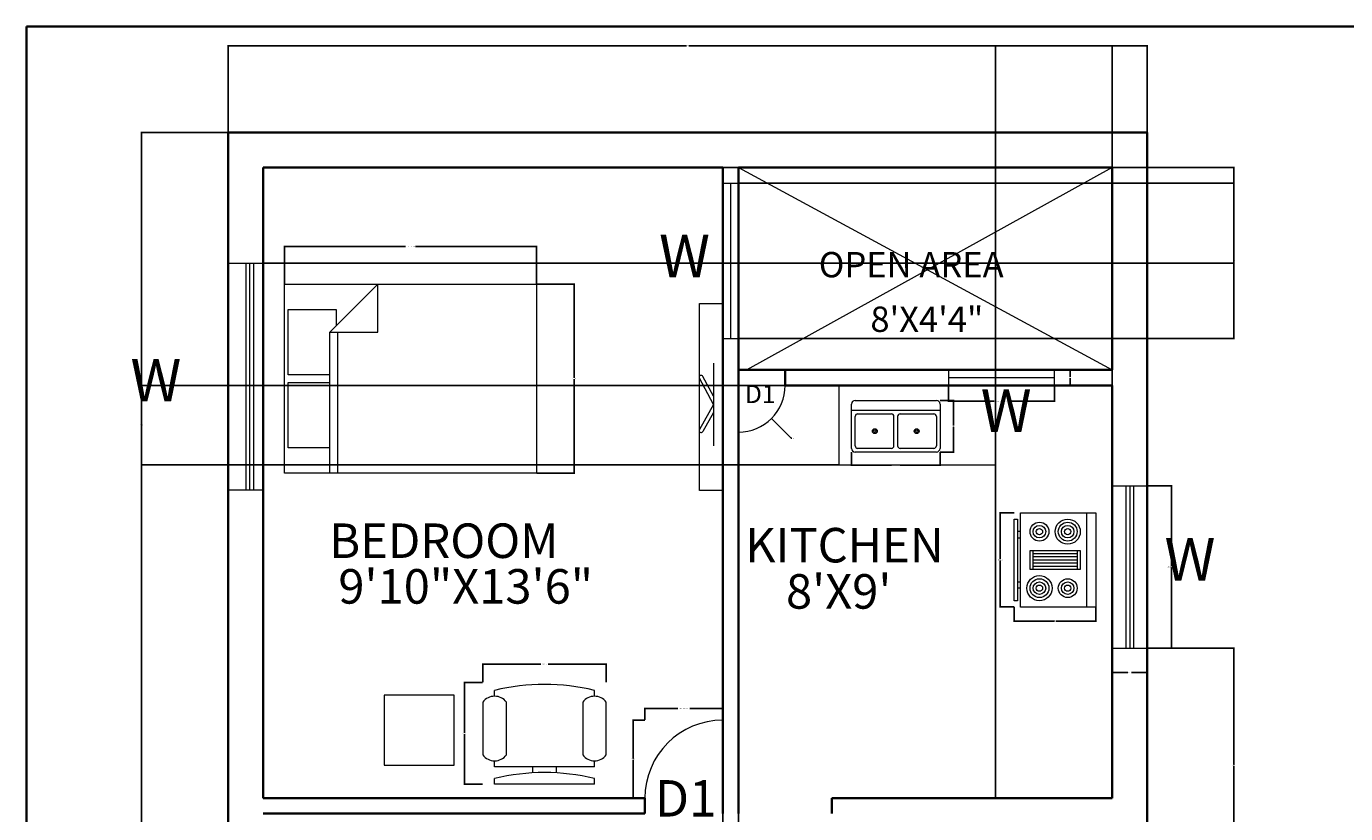
# Model space of a CAD drawing. Units: feet. Extents: x 38163 to 38841, y 65807 to 66292.
# Tile 2 of 3: x 38163 to 38502, y 66090 to 66292. Entities that reach past the tile are written whole.
import ezdxf

# ---------------------------------------------------------------- set-up
doc = ezdxf.new("R2010")
doc.units = ezdxf.units.FT
for name, color, linetype, lineweight in [('A-ANNO-DIMS', 2, 'Continuous', 18), ('A-ANNO-TEXT', 7, 'Continuous', 18), ('A-ANNO-TTLB', 7, 'Continuous', 35), ('A-AREA-IDEN', 7, 'Continuous', 18), ('A-DOOR', 4, 'Continuous', 18), ('A-EQPM', 8, 'Continuous', 18), ('A-FLOR-CASE', 9, 'Continuous', 18), ('A-FLOR-FIXT', 9, 'Continuous', 18), ('A-FLOR-OPEN', 8, 'Continuous', 13), ('A-FURN', 8, 'Continuous', 18), ('A-GLAZ', 4, 'Continuous', 13), ('A-WALL', 7, 'Continuous', 35)]:
    doc.layers.add(name, color=color, linetype=linetype, lineweight=lineweight)
doc.styles.get("Standard").update_dxf_attribs({"font": 'arial.ttf'})
doc.dimstyles.get("Standard").update_dxf_attribs({"dimtxt": 0.18, "dimasz": 0.18, "dimexe": 0.18, "dimexo": 0.0625, "dimgap": 0.09, "dimtad": 0, "dimtih": 1, "dimtoh": 1, "dimdec": 4, "dimzin": 0, "dimdsep": 46, "dimtxsty": 'Standard', "dimcen": 0.09, "dimadec": 0, "dimazin": 0, "dimtfac": 1, "dimtdec": 4, "dimtofl": 0, "dimtmove": 0, "dimatfit": 3, "dimfxl": 1, "dimtolj": 1, "dimtzin": 0, "dimarcsym": 0})

# ---------------------------------------------------------------- blocks, each defined once
blk = doc.blocks.new('Bed - Queen')
for p, q in [((0, -80.00003), (0, 0)), ((0, 0), (59.99999, 0)), ((59.99999, 0), (59.99999, -80.00003)), ((7.99999, -1.2), (28.79998, -1.2)), ((7.99999, -14.4), (7.99999, -1.2)), ((28.79998, -1.2), (28.79998, -14.4)), ((31.19999, -1.2), (51.99999, -1.2)), ((31.19999, -14.4), (31.19999, -1.2)), ((51.99999, -1.2), (51.99999, -16.4)), ((0, -14.4), (44.8, -14.4)), ((59.99999, -29.6), (44.8, -14.4)), ((44.8, -14.4), (44.8, -29.6)), ((51.99999, -16.4), (46.79936, -16.4)), ((44.8, -16.8), (0, -16.8)), ((44.8, -29.6), (59.99999, -29.6)), ((59.99999, -80.00003), (0, -80.00003))]:
    blk.add_line(p, q)
blk = doc.blocks.new('Chair - Desk')
for p, q in [((-8.5, 0), (-8.5, -1)), ((-8.5, 0), (8.5, 0)), ((8.5, 0), (8.5, -1)), ((-2, -3), (-2, -1.9355)), ((2, -1.9576), (2, -3)), ((-8.5, -3), (-8.5, -4)), ((-8.5, -3), (8.5, -3)), ((8.5, -3), (8.5, -4)), ((-10.5, -5), (-10.5, -14)), ((-6.5, -14), (-6.5, -5)), ((6.5, -5), (6.5, -14)), ((10.5, -14), (10.5, -5)), ((-8.5, -15), (-8.5, -16)), ((8.5, -15), (8.5, -16))]:
    blk.add_line(p, q)
for centre, radius, start, end in [((0, 34.625), 36.625, 256.5803, 283.4197), ((-8.5, -6.5), 2.5, 36.8699, 143.1301), ((8.5, -6.5), 2.5, 36.8699, 143.1301), ((-8.5, -12.5), 2.5, 216.8699, 323.1301), ((8.5, -12.5), 2.5, 216.8699, 323.1301), ((0, 19.625), 36.625, 256.5803, 283.4197)]:
    blk.add_arc(centre, radius, start, end)
blk = doc.blocks.new('Range-Oven - 30 in top')
for p, q in [((0, -3), (30, -3)), ((12, -6), (18, -6)), ((13, -20), (13, -6)), ((14, -6), (14, -20)), ((15, -20), (15, -6)), ((16, -6), (16, -20)), ((17, -20), (17, -6)), ((18, -20), (12, -20)), ((6, -24), (6, -25)), ((8, -25), (8, -24)), ((22, -25), (22, -24)), ((24, -24), (24, -25))]:
    blk.add_line(p, q)
for points in [[(0, -24), (0, 0), (30, 0), (30, -24)], [(12, -21), (12, -5), (18, -5), (18, -21)], [(2, -26), (2, -25), (28, -25), (28, -26)]]:
    blk.add_lwpolyline(points, close=True)
for centre, radius in [((6, -9), 4), ((6, -9), 3), ((6, -9), 2), ((6, -9), 1), ((24, -9), 3), ((24, -9), 2), ((24, -9), 1), ((6, -18), 3), ((6, -18), 2), ((24, -18), 4), ((24, -18), 3), ((24, -18), 2), ((6, -18), 1), ((24, -18), 1)]:
    blk.add_circle(centre, radius)
blk = doc.blocks.new('Sink-double - 36 in top')
for p, q in [((-18, -4), (18, -4)), ((-0.75, -18.5), (-0.75, -6.5)), ((0.75, -6.5), (0.75, -18.5))]:
    blk.add_line(p, q)
for points in [[(-16.5, 0), (16.5, 0)], [(-18, -19.5), (-18, -1.5)], [(18, -1.5), (18, -19.5)], [(-16.5, -18.5), (-16.5, -6.5)], [(-15.5, -5.5), (-1.75, -5.5)], [(1.75, -5.5), (15.5, -5.5)], [(16.5, -6.5), (16.5, -18.5)], [(16.5, -21), (-16.5, -21)], [(-1.75, -19.5), (-15.5, -19.5)], [(15.5, -19.5), (1.75, -19.5)]]:
    blk.add_lwpolyline(points)
for centre, radius in [((-8.5, -12.5), 1), ((-8.5, -12.5), 0.5), ((8.5, -12.5), 1), ((8.5, -12.5), 0.5)]:
    blk.add_circle(centre, radius)
for centre, radius, start, end in [((-16.5, -1.5), 1.5, 90, 180), ((16.5, -1.5), 1.5, 0, 90), ((-15.5, -6.5), 1, 90, 180), ((-1.75, -6.5), 1, 0, 90), ((1.75, -6.5), 1, 90, 180), ((15.5, -6.5), 1, 0, 90), ((-16.5, -19.5), 1.5, 180, 270), ((-15.5, -18.5), 1, 180, 270), ((-1.75, -18.5), 1, 270, 0), ((1.75, -18.5), 1, 180, 270), ((15.5, -18.5), 1, 270, 0), ((16.5, -19.5), 1.5, 270, 0)]:
    blk.add_arc(centre, radius, start, end)
blk = doc.blocks.new('DOOR-SWING-20')
blk.add_line((20, 0), (20, 20))
blk.add_arc((20, 0), 20, 90, 180)
blk = doc.blocks.new('TABLE-SQUARE')
for p, q in [((18, 18), (0, 18)), ((0, 18), (0, 0)), ((18, 0), (18, 18)), ((0, 0), (18, 0))]:
    blk.add_line(p, q)
blk = doc.blocks.new('TV-CONSOLE')
for p, q in [((0.06, 48), (6.06, 48)), ((0.06, 0), (0.06, 48)), ((6.06, 48), (6.06, 0)), ((3.68, 32.75), (3.68, 11.44)), ((3.68, 22.09), (0.06, 28.83)), ((3.68, 24.21), (0.94, 29.3)), ((3.68, 22.09), (0.06, 15.67)), ((3.68, 20.06), (0.93, 15.18)), ((6.06, 0), (0.06, 0))]:
    blk.add_line(p, q)
for centre, start, end in [((0.5, 29.07), 28.2522, 208.2522), ((0.5, 15.42), 150.6168, 330.6168)]:
    blk.add_arc(centre, 0.5, start, end)
blk = doc.blocks.new('WIN-SIDE-REAR')
for p, q in [((0, 41.67), (9, 41.67)), ((3.5, 41.67), (3.5, 0)), ((4.5, 41.67), (4.5, 0)), ((5.5, 41.67), (5.5, 0)), ((0, 0), (9, 0))]:
    blk.add_line(p, q)
blk = doc.blocks.new('WIN-LIGHTWELL')
for p, q in [((0, 0), (0, 4)), ((27.16, 0), (27.16, 4)), ((0, 2), (27.16, 2))]:
    blk.add_line(p, q)
blk = doc.blocks.new('LIGHTWELL-CROSS')
for p, q in [((0, 52), (96, 0)), ((96, 52), (2.18, 0))]:
    blk.add_line(p, q)
blk = doc.blocks.new('*D21')
at = {"layer": 'A-ANNO-DIMS', "color": 0, "lineweight": -2, "transparency": 16777216}
for p, q in [((38322.09, 66114.08), (38322.09, 66117.19)), ((38322.27, 66117.01), (38330.52, 66117.01)), ((38341.91, 66117.01), (38333.66, 66117.01)), ((38342.09, 66114.08), (38342.09, 66117.19))]:
    blk.add_line(p, q, dxfattribs=at)
at = {"layer": 'A-ANNO-DIMS', "color": 0, "transparency": 16777216}
for points in [[(38322.27, 66117.04), (38322.27, 66116.98), (38322.09, 66117.01)], [(38341.91, 66117.04), (38341.91, 66116.98), (38342.09, 66117.01)]]:
    blk.add_solid(points, dxfattribs=at)
at = {"layer": 'Defpoints', "color": 0, "transparency": 16777216}
for p in [(38342.09, 66117.01), (38322.09, 66114.01), (38342.09, 66114.01)]:
    blk.add_point(p, dxfattribs=at)
at = {"layer": 'A-ANNO-DIMS', "color": 0, "transparency": 16777216, "insert": (38332.09, 66117.01), "char_height": 0.18, "attachment_point": 5}
blk.add_mtext('\\A1;INTERIOR DOOR 20 TYP.', dxfattribs=at)
blk = doc.blocks.new('*D22')
at = {"layer": 'A-ANNO-DIMS', "color": 0, "lineweight": -2, "transparency": 16777216}
for p, q in [((38322.03, 66114.01), (38318.91, 66114.01)), ((38319.09, 66113.83), (38319.09, 66104.19)), ((38319.09, 66094.19), (38319.09, 66103.83)), ((38322.03, 66094.01), (38318.91, 66094.01))]:
    blk.add_line(p, q, dxfattribs=at)
at = {"layer": 'A-ANNO-DIMS', "color": 0, "transparency": 16777216}
for points in [[(38319.06, 66113.83), (38319.12, 66113.83), (38319.09, 66114.01)], [(38319.06, 66094.19), (38319.12, 66094.19), (38319.09, 66094.01)]]:
    blk.add_solid(points, dxfattribs=at)
at = {"layer": 'Defpoints', "color": 0, "transparency": 16777216}
for p in [(38319.09, 66114.01), (38322.09, 66114.01), (38322.09, 66094.01)]:
    blk.add_point(p, dxfattribs=at)
at = {"layer": 'A-ANNO-DIMS', "color": 0, "transparency": 16777216, "insert": (38319.09, 66104.01), "char_height": 0.18, "attachment_point": 5}
blk.add_mtext('\\A1;20 TYP.', dxfattribs=at)
blk = doc.blocks.new('*D25')
at = {"layer": 'A-ANNO-DIMS', "color": 0, "lineweight": -2, "transparency": 16777216}
for p, q in [((38229.55, 66226.08), (38229.55, 66235.9)), ((38229.73, 66235.72), (38260.59, 66235.72)), ((38294.06, 66235.72), (38263.2, 66235.72)), ((38294.24, 66226.08), (38294.24, 66235.9))]:
    blk.add_line(p, q, dxfattribs=at)
at = {"layer": 'A-ANNO-DIMS', "color": 0, "transparency": 16777216}
for points in [[(38229.73, 66235.75), (38229.73, 66235.69), (38229.55, 66235.72)], [(38294.06, 66235.75), (38294.06, 66235.69), (38294.24, 66235.72)]]:
    blk.add_solid(points, dxfattribs=at)
at = {"layer": 'Defpoints', "color": 0, "transparency": 16777216}
for p in [(38229.55, 66235.72), (38229.55, 66226.02), (38294.24, 66226.02)]:
    blk.add_point(p, dxfattribs=at)
at = {"layer": 'A-ANNO-DIMS', "color": 0, "transparency": 16777216, "insert": (38261.9, 66235.72), "char_height": 0.18, "attachment_point": 5}
blk.add_mtext('\\A1;QUEEN BED 65 TYP.', dxfattribs=at)
blk = doc.blocks.new('*D26')
at = {"layer": 'A-ANNO-DIMS', "color": 0, "lineweight": -2, "transparency": 16777216}
for p, q in [((38294.31, 66226.02), (38304.13, 66226.02)), ((38303.95, 66225.84), (38303.95, 66201.94)), ((38303.95, 66177.68), (38303.95, 66201.58)), ((38294.31, 66177.5), (38304.13, 66177.5))]:
    blk.add_line(p, q, dxfattribs=at)
at = {"layer": 'A-ANNO-DIMS', "color": 0, "transparency": 16777216}
for points in [[(38303.92, 66225.84), (38303.98, 66225.84), (38303.95, 66226.02)], [(38303.92, 66177.68), (38303.98, 66177.68), (38303.95, 66177.5)]]:
    blk.add_solid(points, dxfattribs=at)
at = {"layer": 'Defpoints', "color": 0, "transparency": 16777216}
for p in [(38294.24, 66226.02), (38303.95, 66226.02), (38294.24, 66177.5)]:
    blk.add_point(p, dxfattribs=at)
at = {"layer": 'A-ANNO-DIMS', "color": 0, "transparency": 16777216, "insert": (38303.95, 66201.76), "char_height": 0.18, "attachment_point": 5}
blk.add_mtext('\\A1;49 TYP.', dxfattribs=at)
blk = doc.blocks.new('*D27')
at = {"layer": 'A-ANNO-DIMS', "color": 0, "lineweight": -2, "transparency": 16777216}
for p, q in [((38280.48, 66123.75), (38280.48, 66128.61)), ((38280.66, 66128.43), (38295.36, 66128.43)), ((38311.97, 66128.43), (38297.27, 66128.43)), ((38312.15, 66123.75), (38312.15, 66128.61))]:
    blk.add_line(p, q, dxfattribs=at)
at = {"layer": 'A-ANNO-DIMS', "color": 0, "transparency": 16777216}
for points in [[(38280.66, 66128.46), (38280.66, 66128.4), (38280.48, 66128.43)], [(38311.97, 66128.46), (38311.97, 66128.4), (38312.15, 66128.43)]]:
    blk.add_solid(points, dxfattribs=at)
at = {"layer": 'Defpoints', "color": 0, "transparency": 16777216}
for p in [(38280.48, 66128.43), (38280.48, 66123.68), (38312.15, 66123.68)]:
    blk.add_point(p, dxfattribs=at)
at = {"layer": 'A-ANNO-DIMS', "color": 0, "transparency": 16777216, "insert": (38296.32, 66128.43), "char_height": 0.18, "attachment_point": 5}
blk.add_mtext('\\A1;CHAIR 32 TYP.', dxfattribs=at)
blk = doc.blocks.new('*D28')
at = {"layer": 'A-ANNO-DIMS', "color": 0, "lineweight": -2, "transparency": 16777216}
for p, q in [((38280.42, 66123.68), (38275.55, 66123.68)), ((38275.73, 66123.5), (38275.73, 66110.8)), ((38275.73, 66097.73), (38275.73, 66110.43)), ((38280.42, 66097.55), (38275.55, 66097.55))]:
    blk.add_line(p, q, dxfattribs=at)
at = {"layer": 'A-ANNO-DIMS', "color": 0, "transparency": 16777216}
for points in [[(38275.7, 66123.5), (38275.76, 66123.5), (38275.73, 66123.68)], [(38275.7, 66097.73), (38275.76, 66097.73), (38275.73, 66097.55)]]:
    blk.add_solid(points, dxfattribs=at)
at = {"layer": 'Defpoints', "color": 0, "transparency": 16777216}
for p in [(38280.48, 66123.68), (38275.73, 66097.55), (38280.48, 66097.55)]:
    blk.add_point(p, dxfattribs=at)
at = {"layer": 'A-ANNO-DIMS', "color": 0, "transparency": 16777216, "insert": (38275.73, 66110.61), "char_height": 0.18, "attachment_point": 5}
blk.add_mtext('\\A1;26 TYP.', dxfattribs=at)
blk = doc.blocks.new('*D45')
at = {"layer": 'A-ANNO-DIMS', "color": 0, "lineweight": -2, "transparency": 16777216}
for p, q in [((38451.15, 66174.22), (38457.52, 66174.22)), ((38457.34, 66174.04), (38457.34, 66153.56)), ((38457.34, 66132.72), (38457.34, 66153.2)), ((38451.15, 66132.54), (38457.52, 66132.54))]:
    blk.add_line(p, q, dxfattribs=at)
at = {"layer": 'A-ANNO-DIMS', "color": 0, "transparency": 16777216}
for points in [[(38457.31, 66174.04), (38457.37, 66174.04), (38457.34, 66174.22)], [(38457.31, 66132.72), (38457.37, 66132.72), (38457.34, 66132.54)]]:
    blk.add_solid(points, dxfattribs=at)
at = {"layer": 'Defpoints', "color": 0, "transparency": 16777216}
for p in [(38451.09, 66174.22), (38457.34, 66174.22), (38451.09, 66132.54)]:
    blk.add_point(p, dxfattribs=at)
at = {"layer": 'A-ANNO-DIMS', "color": 0, "transparency": 16777216, "insert": (38457.34, 66153.38), "char_height": 0.18, "attachment_point": 5}
blk.add_mtext('\\A1;REAR WINDOW 42 TYP.', dxfattribs=at)
blk = doc.blocks.new('*D46')
at = {"layer": 'A-ANNO-DIMS', "color": 0, "lineweight": -2, "transparency": 16777216}
for p, q in [((38442.09, 66132.48), (38442.09, 66126.11)), ((38451.09, 66132.48), (38451.09, 66126.11)), ((38442.27, 66126.29), (38446.13, 66126.29)), ((38450.91, 66126.29), (38447.05, 66126.29))]:
    blk.add_line(p, q, dxfattribs=at)
at = {"layer": 'A-ANNO-DIMS', "color": 0, "transparency": 16777216}
for points in [[(38442.27, 66126.32), (38442.27, 66126.26), (38442.09, 66126.29)], [(38450.91, 66126.32), (38450.91, 66126.26), (38451.09, 66126.29)]]:
    blk.add_solid(points, dxfattribs=at)
at = {"layer": 'Defpoints', "color": 0, "transparency": 16777216}
for p in [(38442.09, 66132.54), (38451.09, 66132.54), (38451.09, 66126.29)]:
    blk.add_point(p, dxfattribs=at)
at = {"layer": 'A-ANNO-DIMS', "color": 0, "transparency": 16777216, "insert": (38446.59, 66126.29), "char_height": 0.18, "attachment_point": 5}
blk.add_mtext('\\A1;9 TYP.', dxfattribs=at)
blk = doc.blocks.new('*D49')
at = {"layer": 'A-ANNO-DIMS', "color": 0, "lineweight": -2, "transparency": 16777216}
for p, q in [((38400.09, 66199.95), (38400.09, 66195.76)), ((38427.25, 66199.95), (38427.25, 66195.76)), ((38400.27, 66195.94), (38411.81, 66195.94)), ((38427.07, 66195.94), (38415.53, 66195.94))]:
    blk.add_line(p, q, dxfattribs=at)
at = {"layer": 'A-ANNO-DIMS', "color": 0, "transparency": 16777216}
for points in [[(38400.27, 66195.97), (38400.27, 66195.91), (38400.09, 66195.94)], [(38427.07, 66195.97), (38427.07, 66195.91), (38427.25, 66195.94)]]:
    blk.add_solid(points, dxfattribs=at)
at = {"layer": 'Defpoints', "color": 0, "transparency": 16777216}
for p in [(38400.09, 66200.01), (38427.25, 66200.01), (38427.25, 66195.94)]:
    blk.add_point(p, dxfattribs=at)
at = {"layer": 'A-ANNO-DIMS', "color": 0, "transparency": 16777216, "insert": (38413.67, 66195.94), "char_height": 0.18, "attachment_point": 5}
blk.add_mtext('\\A1;LIGHTWELL WINDOW 27 TYP.', dxfattribs=at)
blk = doc.blocks.new('*D50')
at = {"layer": 'A-ANNO-DIMS', "color": 0, "lineweight": -2, "transparency": 16777216}
for p, q in [((38427.31, 66204.01), (38431.5, 66204.01)), ((38431.32, 66203.83), (38431.32, 66202.19)), ((38431.32, 66200.19), (38431.32, 66201.83)), ((38427.31, 66200.01), (38431.5, 66200.01))]:
    blk.add_line(p, q, dxfattribs=at)
at = {"layer": 'A-ANNO-DIMS', "color": 0, "transparency": 16777216}
for points in [[(38431.29, 66203.83), (38431.35, 66203.83), (38431.32, 66204.01)], [(38431.29, 66200.19), (38431.35, 66200.19), (38431.32, 66200.01)]]:
    blk.add_solid(points, dxfattribs=at)
at = {"layer": 'Defpoints', "color": 0, "transparency": 16777216}
for p in [(38427.25, 66204.01), (38431.32, 66204.01), (38427.25, 66200.01)]:
    blk.add_point(p, dxfattribs=at)
at = {"layer": 'A-ANNO-DIMS', "color": 0, "transparency": 16777216, "insert": (38431.32, 66202.01), "char_height": 0.18, "attachment_point": 5}
blk.add_mtext('\\A1;4 TYP.', dxfattribs=at)
blk = doc.blocks.new('*D53')
at = {"layer": 'A-ANNO-DIMS', "color": 0, "lineweight": -2, "transparency": 16777216}
for p, q in [((38416.89, 66167.28), (38413.14, 66167.28)), ((38413.32, 66167.1), (38413.32, 66155.37)), ((38413.32, 66143.27), (38413.32, 66155)), ((38416.89, 66143.09), (38413.14, 66143.09))]:
    blk.add_line(p, q, dxfattribs=at)
at = {"layer": 'A-ANNO-DIMS', "color": 0, "transparency": 16777216}
for points in [[(38413.29, 66167.1), (38413.35, 66167.1), (38413.32, 66167.28)], [(38413.29, 66143.27), (38413.35, 66143.27), (38413.32, 66143.09)]]:
    blk.add_solid(points, dxfattribs=at)
at = {"layer": 'Defpoints', "color": 0, "transparency": 16777216}
for p in [(38416.95, 66167.28), (38413.32, 66143.09), (38416.95, 66143.09)]:
    blk.add_point(p, dxfattribs=at)
at = {"layer": 'A-ANNO-DIMS', "color": 0, "transparency": 16777216, "insert": (38413.32, 66155.18), "char_height": 0.18, "attachment_point": 5}
blk.add_mtext('\\A1;RANGE 24', dxfattribs=at)
blk = doc.blocks.new('*D54')
at = {"layer": 'A-ANNO-DIMS', "color": 0, "lineweight": -2, "transparency": 16777216}
for p, q in [((38416.95, 66143.02), (38416.95, 66139.28)), ((38437.92, 66143.02), (38437.92, 66139.28)), ((38417.13, 66139.46), (38427.23, 66139.46)), ((38437.74, 66139.46), (38427.64, 66139.46))]:
    blk.add_line(p, q, dxfattribs=at)
at = {"layer": 'A-ANNO-DIMS', "color": 0, "transparency": 16777216}
for points in [[(38417.13, 66139.49), (38417.13, 66139.43), (38416.95, 66139.46)], [(38437.74, 66139.49), (38437.74, 66139.43), (38437.92, 66139.46)]]:
    blk.add_solid(points, dxfattribs=at)
at = {"layer": 'Defpoints', "color": 0, "transparency": 16777216}
for p in [(38416.95, 66143.09), (38437.92, 66143.09), (38437.92, 66139.46)]:
    blk.add_point(p, dxfattribs=at)
at = {"layer": 'A-ANNO-DIMS', "color": 0, "transparency": 16777216, "insert": (38427.43, 66139.46), "char_height": 0.18, "attachment_point": 5}
blk.add_mtext('\\A1;21', dxfattribs=at)
blk = doc.blocks.new('*D55')
at = {"layer": 'A-ANNO-DIMS', "color": 0, "lineweight": -2, "transparency": 16777216}
for p, q in [((38375.14, 66182.83), (38375.14, 66179.31)), ((38397.88, 66182.83), (38397.88, 66179.31)), ((38375.32, 66179.49), (38385.42, 66179.49)), ((38397.7, 66179.49), (38387.61, 66179.49))]:
    blk.add_line(p, q, dxfattribs=at)
at = {"layer": 'A-ANNO-DIMS', "color": 0, "transparency": 16777216}
for points in [[(38375.32, 66179.52), (38375.32, 66179.46), (38375.14, 66179.49)], [(38397.7, 66179.52), (38397.7, 66179.46), (38397.88, 66179.49)]]:
    blk.add_solid(points, dxfattribs=at)
at = {"layer": 'Defpoints', "color": 0, "transparency": 16777216}
for p in [(38375.14, 66182.9), (38397.88, 66182.9), (38397.88, 66179.49)]:
    blk.add_point(p, dxfattribs=at)
at = {"layer": 'A-ANNO-DIMS', "color": 0, "transparency": 16777216, "insert": (38386.51, 66179.49), "char_height": 0.18, "attachment_point": 5}
blk.add_mtext('\\A1;DOUBLE SINK 23', dxfattribs=at)
blk = doc.blocks.new('*D56')
at = {"layer": 'A-ANNO-DIMS', "color": 0, "lineweight": -2, "transparency": 16777216}
for p, q in [((38397.94, 66196.16), (38401.47, 66196.16)), ((38401.29, 66195.98), (38401.29, 66189.71)), ((38401.29, 66183.08), (38401.29, 66189.35)), ((38397.94, 66182.9), (38401.47, 66182.9))]:
    blk.add_line(p, q, dxfattribs=at)
at = {"layer": 'A-ANNO-DIMS', "color": 0, "transparency": 16777216}
for points in [[(38401.26, 66195.98), (38401.32, 66195.98), (38401.29, 66196.16)], [(38401.26, 66183.08), (38401.32, 66183.08), (38401.29, 66182.9)]]:
    blk.add_solid(points, dxfattribs=at)
at = {"layer": 'Defpoints', "color": 0, "transparency": 16777216}
for p in [(38397.88, 66196.16), (38401.29, 66196.16), (38397.88, 66182.9)]:
    blk.add_point(p, dxfattribs=at)
at = {"layer": 'A-ANNO-DIMS', "color": 0, "transparency": 16777216, "insert": (38401.29, 66189.53), "char_height": 0.18, "attachment_point": 5}
blk.add_mtext('\\A1;13', dxfattribs=at)
blk = doc.blocks.new('*D57')
at = {"layer": 'A-ANNO-DIMS', "color": 0, "lineweight": -2, "transparency": 16777216}
for p, q in [((38215.09, 66265.08), (38215.09, 66287.44)), ((38215.27, 66287.26), (38332.8, 66287.26)), ((38450.91, 66287.26), (38333.38, 66287.26)), ((38451.09, 66265.08), (38451.09, 66287.44))]:
    blk.add_line(p, q, dxfattribs=at)
at = {"layer": 'A-ANNO-DIMS', "color": 0, "transparency": 16777216}
for points in [[(38215.27, 66287.29), (38215.27, 66287.23), (38215.09, 66287.26)], [(38450.91, 66287.29), (38450.91, 66287.23), (38451.09, 66287.26)]]:
    blk.add_solid(points, dxfattribs=at)
at = {"layer": 'Defpoints', "color": 0, "transparency": 16777216}
for p in [(38451.09, 66287.26), (38215.09, 66265.01), (38451.09, 66265.01)]:
    blk.add_point(p, dxfattribs=at)
at = {"layer": 'A-ANNO-DIMS', "color": 0, "transparency": 16777216, "insert": (38333.09, 66287.26), "char_height": 0.18, "attachment_point": 5}
blk.add_mtext('\\A1;236', dxfattribs=at)
blk = doc.blocks.new('*D58')
at = {"layer": 'A-ANNO-DIMS', "color": 0, "lineweight": -2, "transparency": 16777216}
for p, q in [((38215.03, 66265.01), (38192.66, 66265.01)), ((38192.84, 66264.83), (38192.84, 66087.19)), ((38192.84, 65909.19), (38192.84, 66086.83)), ((38215.03, 65909.01), (38192.66, 65909.01))]:
    blk.add_line(p, q, dxfattribs=at)
at = {"layer": 'A-ANNO-DIMS', "color": 0, "transparency": 16777216}
for points in [[(38192.81, 66264.83), (38192.87, 66264.83), (38192.84, 66265.01)], [(38192.81, 65909.19), (38192.87, 65909.19), (38192.84, 65909.01)]]:
    blk.add_solid(points, dxfattribs=at)
at = {"layer": 'Defpoints', "color": 0, "transparency": 16777216}
for p in [(38192.84, 66265.01), (38215.09, 66265.01), (38215.09, 65909.01)]:
    blk.add_point(p, dxfattribs=at)
at = {"layer": 'A-ANNO-DIMS', "color": 0, "transparency": 16777216, "insert": (38192.84, 66087.01), "char_height": 0.18, "attachment_point": 5}
blk.add_mtext('\\A1;356', dxfattribs=at)
blk = doc.blocks.new('*D64')
at = {"layer": 'A-ANNO-DIMS', "color": 0, "lineweight": -2, "transparency": 16777216}
for p, q in [((38451.15, 66132.54), (38473.52, 66132.54)), ((38473.34, 66132.36), (38473.34, 66102.65)), ((38473.34, 66072.57), (38473.34, 66102.29)), ((38451.15, 66072.39), (38473.52, 66072.39))]:
    blk.add_line(p, q, dxfattribs=at)
at = {"layer": 'A-ANNO-DIMS', "color": 0, "transparency": 16777216}
for points in [[(38473.31, 66132.36), (38473.37, 66132.36), (38473.34, 66132.54)], [(38473.31, 66072.57), (38473.37, 66072.57), (38473.34, 66072.39)]]:
    blk.add_solid(points, dxfattribs=at)
at = {"layer": 'Defpoints', "color": 0, "transparency": 16777216}
for p in [(38451.09, 66132.54), (38473.34, 66132.54), (38451.09, 66072.39)]:
    blk.add_point(p, dxfattribs=at)
at = {"layer": 'A-ANNO-DIMS', "color": 0, "transparency": 16777216, "insert": (38473.34, 66102.47), "char_height": 0.18, "attachment_point": 5}
blk.add_mtext('\\A1;60.15', dxfattribs=at)
blk = doc.blocks.new('*D65')
at = {"layer": 'A-ANNO-DIMS', "color": 0, "lineweight": -2, "transparency": 16777216}
for p, q in [((38224.15, 66256.01), (38473.52, 66256.01)), ((38473.34, 66255.83), (38473.34, 66243.88)), ((38473.34, 66231.56), (38473.34, 66243.52)), ((38224.15, 66231.38), (38473.52, 66231.38))]:
    blk.add_line(p, q, dxfattribs=at)
at = {"layer": 'A-ANNO-DIMS', "color": 0, "transparency": 16777216}
for points in [[(38473.31, 66255.83), (38473.37, 66255.83), (38473.34, 66256.01)], [(38473.31, 66231.56), (38473.37, 66231.56), (38473.34, 66231.38)]]:
    blk.add_solid(points, dxfattribs=at)
at = {"layer": 'Defpoints', "color": 0, "transparency": 16777216}
for p in [(38224.09, 66256.01), (38224.09, 66231.38), (38473.34, 66231.38)]:
    blk.add_point(p, dxfattribs=at)
at = {"layer": 'A-ANNO-DIMS', "color": 0, "transparency": 16777216, "insert": (38473.34, 66243.7), "char_height": 0.18, "attachment_point": 5}
blk.add_mtext('\\A1;24.63', dxfattribs=at)
blk = doc.blocks.new('*D69')
at = {"layer": 'A-ANNO-DIMS', "color": 0, "lineweight": -2, "transparency": 16777216}
for p, q in [((38346.15, 66252), (38473.52, 66252)), ((38473.34, 66251.82), (38473.34, 66232.22)), ((38473.34, 66212.26), (38473.34, 66231.86)), ((38346.15, 66212.08), (38473.52, 66212.08))]:
    blk.add_line(p, q, dxfattribs=at)
at = {"layer": 'A-ANNO-DIMS', "color": 0, "transparency": 16777216}
for points in [[(38473.31, 66251.82), (38473.37, 66251.82), (38473.34, 66252)], [(38473.31, 66212.26), (38473.37, 66212.26), (38473.34, 66212.08)]]:
    blk.add_solid(points, dxfattribs=at)
at = {"layer": 'Defpoints', "color": 0, "transparency": 16777216}
for p in [(38346.09, 66252), (38346.09, 66212.08), (38473.34, 66212.08)]:
    blk.add_point(p, dxfattribs=at)
at = {"layer": 'A-ANNO-DIMS', "color": 0, "transparency": 16777216, "insert": (38473.34, 66232.04), "char_height": 0.18, "attachment_point": 5}
blk.add_mtext('\\A1;39.92', dxfattribs=at)
blk = doc.blocks.new('*D75')
at = {"layer": 'A-ANNO-DIMS', "color": 0, "lineweight": -2, "transparency": 16777216}
for p, q in [((38412.09, 66094.08), (38412.09, 66287.44)), ((38412.27, 66287.26), (38426.87, 66287.26)), ((38441.91, 66287.26), (38427.31, 66287.26)), ((38442.09, 66094.08), (38442.09, 66287.44))]:
    blk.add_line(p, q, dxfattribs=at)
at = {"layer": 'A-ANNO-DIMS', "color": 0, "transparency": 16777216}
for points in [[(38412.27, 66287.29), (38412.27, 66287.23), (38412.09, 66287.26)], [(38441.91, 66287.29), (38441.91, 66287.23), (38442.09, 66287.26)]]:
    blk.add_solid(points, dxfattribs=at)
at = {"layer": 'Defpoints', "color": 0, "transparency": 16777216}
for p in [(38442.09, 66287.26), (38412.09, 66094.01), (38442.09, 66094.01)]:
    blk.add_point(p, dxfattribs=at)
at = {"layer": 'A-ANNO-DIMS', "color": 0, "transparency": 16777216, "insert": (38427.09, 66287.26), "char_height": 0.18, "attachment_point": 5}
blk.add_mtext('\\A1;30', dxfattribs=at)
blk = doc.blocks.new('*D76')
at = {"layer": 'A-ANNO-DIMS', "color": 0, "lineweight": -2, "transparency": 16777216}
for p, q in [((38371.87, 66200.01), (38192.66, 66200.01)), ((38192.84, 66199.83), (38192.84, 66189.99)), ((38192.84, 66179.78), (38192.84, 66189.63)), ((38371.87, 66179.6), (38192.66, 66179.6))]:
    blk.add_line(p, q, dxfattribs=at)
at = {"layer": 'A-ANNO-DIMS', "color": 0, "transparency": 16777216}
for points in [[(38192.81, 66199.83), (38192.87, 66199.83), (38192.84, 66200.01)], [(38192.81, 66179.78), (38192.87, 66179.78), (38192.84, 66179.6)]]:
    blk.add_solid(points, dxfattribs=at)
at = {"layer": 'Defpoints', "color": 0, "transparency": 16777216}
for p in [(38192.84, 66200.01), (38371.93, 66200.01), (38371.93, 66179.6)]:
    blk.add_point(p, dxfattribs=at)
at = {"layer": 'A-ANNO-DIMS', "color": 0, "transparency": 16777216, "insert": (38192.84, 66189.81), "char_height": 0.18, "attachment_point": 5}
blk.add_mtext('\\A1;20.41', dxfattribs=at)
blk = doc.blocks.new('*D80')
at = {"layer": 'A-ANNO-DIMS', "color": 0, "lineweight": -2, "transparency": 16777216}
for p, q in [((38342.09, 66255.95), (38342.09, 65886.58)), ((38346.09, 66255.95), (38346.09, 65886.58)), ((38342.27, 65886.76), (38343.94, 65886.76)), ((38345.91, 65886.76), (38344.24, 65886.76))]:
    blk.add_line(p, q, dxfattribs=at)
at = {"layer": 'A-ANNO-DIMS', "color": 0, "transparency": 16777216}
for points in [[(38342.27, 65886.79), (38342.27, 65886.73), (38342.09, 65886.76)], [(38345.91, 65886.79), (38345.91, 65886.73), (38346.09, 65886.76)]]:
    blk.add_solid(points, dxfattribs=at)
at = {"layer": 'Defpoints', "color": 0, "transparency": 16777216}
for p in [(38342.09, 66256.01), (38346.09, 66256.01), (38346.09, 65886.76)]:
    blk.add_point(p, dxfattribs=at)
at = {"layer": 'A-ANNO-DIMS', "color": 0, "transparency": 16777216, "insert": (38344.09, 65886.76), "char_height": 0.18, "attachment_point": 5}
blk.add_mtext('\\A1;4', dxfattribs=at)
blk = doc.blocks.new('*D81')
at = {"layer": 'A-ANNO-DIMS', "color": 0, "lineweight": -2, "transparency": 16777216}
for p, q in [((38346, 66200.01), (38346.18, 66200.01)), ((38346.09, 66199.92), (38346.09, 66200.1)), ((38359.67, 66186.44), (38354.7, 66191.4)), ((38359.85, 66186.44), (38359.67, 66186.44))]:
    blk.add_line(p, q, dxfattribs=at)
at = {"layer": 'A-ANNO-DIMS', "color": 0, "transparency": 16777216}
blk.add_solid([(38354.73, 66191.42), (38354.68, 66191.38), (38354.58, 66191.53)], dxfattribs=at)
at = {"layer": 'Defpoints', "color": 0, "transparency": 16777216}
for p in [(38346.09, 66200.01), (38354.58, 66191.53)]:
    blk.add_point(p, dxfattribs=at)
at = {"layer": 'A-ANNO-DIMS', "color": 0, "transparency": 16777216, "insert": (38360.15, 66186.44), "char_height": 0.18, "attachment_point": 5}
blk.add_mtext('\\A1;R12', dxfattribs=at)

msp = doc.modelspace()

# ---------------------------------------------------------------- linework, layer by layer
at = {"layer": 'A-ANNO-TTLB'}
msp.add_lwpolyline([(38163.261, 66292.238), (38840.784, 66292.238), (38840.784, 65806.731), (38163.261, 65806.731)], close=True, dxfattribs=at)
at = {"layer": 'A-DOOR'}
msp.add_line((38346.092, 66200.013), (38346.092, 66188.013), dxfattribs=at)
msp.add_arc((38346.092, 66200.013), 12, 270, 0, dxfattribs=at)
at = {"layer": 'A-FLOR-CASE'}
for p, q in [((38371.93, 66200.013), (38371.93, 66179.604)), ((38371.93, 66179.604), (38412.092, 66179.604)), ((38412.092, 66179.604), (38412.092, 66094.013))]:
    msp.add_line(p, q, dxfattribs=at)
at = {"layer": 'A-GLAZ'}
for p, q in [((38342.092, 66252.001), (38346.092, 66252.001)), ((38344.092, 66252.001), (38344.092, 66212.078)), ((38215.092, 66231.382), (38224.092, 66231.382)), ((38219.592, 66231.382), (38219.592, 66173.187)), ((38220.592, 66231.382), (38220.592, 66173.187)), ((38221.592, 66231.382), (38221.592, 66173.187)), ((38342.092, 66212.078), (38346.092, 66212.078)), ((38215.092, 66173.187), (38224.092, 66173.187))]:
    msp.add_line(p, q, dxfattribs=at)
at = {"layer": 'A-WALL'}
for p, q in [((38215.092, 66265.013), (38451.092, 66265.013)), ((38215.092, 65909.013), (38215.092, 66265.013)), ((38346.092, 66265.013), (38451.092, 66265.013)), ((38451.092, 66265.013), (38451.092, 65909.013)), ((38224.092, 66256.013), (38342.092, 66256.013)), ((38224.092, 66094.013), (38224.092, 66256.013)), ((38342.092, 66256.013), (38342.092, 66090.013)), ((38346.092, 66256.013), (38346.092, 66090.013)), ((38346.092, 66256.013), (38442.092, 66256.013)), ((38442.092, 66256.013), (38442.092, 66204.013)), ((38358.092, 66204.013), (38346.092, 66204.013)), ((38442.092, 66204.013), (38358.092, 66204.013)), ((38358.092, 66200.013), (38358.092, 66204.013)), ((38442.092, 66200.013), (38358.092, 66200.013)), ((38442.092, 66200.013), (38442.092, 66094.013)), ((38451.092, 66200.013), (38451.092, 66094.013)), ((38322.092, 66094.013), (38224.092, 66094.013)), ((38322.092, 66094.013), (38322.092, 66090.013)), ((38442.092, 66094.013), (38370.092, 66094.013)), ((38370.092, 66094.013), (38370.092, 66090.013)), ((38322.092, 66090.013), (38224.092, 66090.013))]:
    msp.add_line(p, q, dxfattribs=at)

# ---------------------------------------------------------------- block references
at = {"layer": 'A-DOOR'}
msp.add_blockref('DOOR-SWING-20', (38322.092, 66094.013), dxfattribs=at)
at = {"layer": 'A-EQPM', "xscale": 0.8065686905678981, "yscale": 0.8065686905678981, "zscale": 0.8065686905678981, "rotation": 270}
msp.add_blockref('Range-Oven - 30 in top', (38437.92, 66167.283), dxfattribs=at)
at = {"layer": 'A-FLOR-FIXT', "xscale": 0.6316563595254492, "yscale": 0.6316563595254492, "zscale": 0.6316563595254492}
msp.add_blockref('Sink-double - 36 in top', (38386.51, 66196.162), dxfattribs=at)
at = {"layer": 'A-FLOR-OPEN'}
msp.add_blockref('LIGHTWELL-CROSS', (38346.092, 66204.013), dxfattribs=at)
at = {"layer": 'A-FURN'}
for name, p, xscale, yscale, zscale, rotation in [('Bed - Queen', (38229.547, 66177.497), 0.8087141965759899, 0.8087141965759899, 0.8087141965759899, 90), ('Chair - Desk', (38296.318, 66097.546), 1.507967457796497, 1.507967457796497, 1.507967457796497, 180)]:
    msp.add_blockref(name, p, dxfattribs=dict(at, xscale=xscale, yscale=yscale, zscale=zscale, rotation=rotation))
for name, p in [('TV-CONSOLE', (38336.029, 66173.013)), ('TABLE-SQUARE', (38255.096, 66102.477))]:
    msp.add_blockref(name, p, dxfattribs=at)
at = {"layer": 'A-GLAZ'}
for name, p in [('WIN-LIGHTWELL', (38400.092, 66200.013)), ('WIN-SIDE-REAR', (38442.092, 66132.544))]:
    msp.add_blockref(name, p, dxfattribs=at)

# ---------------------------------------------------------------- texts
at = {"layer": 'A-ANNO-TEXT'}
for s, height, p in [('W', 10.93, (38325.718, 66227.769)), ('W', 10.93, (38189.976, 66195.889)), ('D1', 4.6399, (38347.773, 66195.477)), ('W', 10.93, (38408.313, 66188.056)), ('W', 10.93, (38455.51, 66149.894)), ('D1', 9.3586, (38324.641, 66089.25))]:
    msp.add_text(s, height=height, dxfattribs=at).set_placement(p)
at = {"layer": 'A-AREA-IDEN'}
for s, height, p in [('OPEN AREA', 6.5041, (38366.735, 66227.779)), ('8\'X4\'4"', 6.5041, (38379.999, 66213.757)), ('BEDROOM', 8.8696, (38241.027, 66155.68)), ('KITCHEN', 8.8696, (38347.84, 66154.535)), ('9\'10"X13\'6"', 8.86963, (38243.361, 66143.953)), ("8'X9'", 8.8696, (38358.31, 66142.66))]:
    msp.add_text(s, height=height, dxfattribs=at).set_placement(p)

# ---------------------------------------------------------------- dimensions: what is measured, and where the dimension line sits
at = {"layer": 'A-ANNO-DIMS'}
for base, p1, p2, picture, middle in [((38451.092, 66287.263), (38215.092, 66265.013), (38451.092, 66265.013), '*D57', (38333.092, 66287.263)), ((38442.092, 66287.263), (38412.092, 66094.013), (38442.092, 66094.013), '*D75', (38427.092, 66287.263)), ((38346.092, 65886.763), (38342.092, 66256.013), (38346.092, 66256.013), '*D80', (38344.092, 65886.763)), ((38437.92, 66139.456), (38416.949, 66143.086), (38437.92, 66143.086), '*D54', (38427.434, 66139.456))]:
    dim = msp.add_linear_dim(base=base, p1=p1, p2=p2, dimstyle='Standard', override={"dimdec": 0, "dimlfac": 1, "dimrnd": 0, "dimzin": 0, "dimdsep": 46, "dimlunit": 2}, dxfattribs=at)
    dim.commit()
    dim.dimension.update_dxf_attribs({"geometry": picture, "text_midpoint": middle})
for base, p1, p2, override, picture, middle in [((38192.842, 66265.013), (38215.092, 65909.013), (38215.092, 66265.013), {"dimdec": 0, "dimlfac": 1, "dimrnd": 0, "dimzin": 0, "dimdsep": 46, "dimlunit": 2}, '*D58', (38192.842, 66087.013)), ((38473.342, 66231.382), (38224.092, 66256.013), (38224.092, 66231.382), {"dimdec": 2, "dimlfac": 1, "dimrnd": 0, "dimzin": 0, "dimdsep": 46, "dimlunit": 2}, '*D65', (38473.342, 66243.697)), ((38473.342, 66212.078), (38346.092, 66252.001), (38346.092, 66212.078), {"dimdec": 2, "dimlfac": 1, "dimrnd": 0, "dimzin": 0, "dimdsep": 46, "dimlunit": 2}, '*D69', (38473.342, 66232.04)), ((38192.842, 66200.013), (38371.93, 66179.604), (38371.93, 66200.013), {"dimdec": 2, "dimlfac": 1, "dimrnd": 0, "dimzin": 0, "dimdsep": 46, "dimlunit": 2}, '*D76', (38192.842, 66189.808)), ((38401.291, 66196.162), (38397.88, 66182.897), (38397.88, 66196.162), {"dimdec": 0, "dimlfac": 1, "dimrnd": 0, "dimzin": 0, "dimdsep": 46, "dimlunit": 2}, '*D56', (38401.291, 66189.529)), ((38473.342, 66132.544), (38451.092, 66072.393), (38451.092, 66132.544), {"dimdec": 2, "dimlfac": 1, "dimrnd": 0, "dimzin": 0, "dimdsep": 46, "dimlunit": 2}, '*D64', (38473.342, 66102.469))]:
    dim = msp.add_linear_dim(base=base, p1=p1, p2=p2, angle=90, dimstyle='Standard', override=override, dxfattribs=at)
    dim.commit()
    dim.dimension.update_dxf_attribs({"geometry": picture, "text_midpoint": middle})
for base, p1, p2, angle, text, picture, middle in [((38229.547, 66235.725), (38294.244, 66226.02), (38229.547, 66226.02), 180, 'QUEEN BED <> TYP.', '*D25', (38261.895, 66235.725)), ((38303.949, 66226.02), (38294.244, 66177.497), (38294.244, 66226.02), 90, '<> TYP.', '*D26', (38303.949, 66201.759)), ((38431.325, 66204.013), (38427.251, 66200.013), (38427.251, 66204.013), 90, '<> TYP.', '*D50', (38431.325, 66202.013)), ((38457.342, 66174.216), (38451.092, 66132.544), (38451.092, 66174.216), 90, 'REAR WINDOW <> TYP.', '*D45', (38457.342, 66153.38)), ((38413.319, 66143.086), (38416.949, 66167.283), (38416.949, 66143.086), 270, 'RANGE <>', '*D53', (38413.319, 66155.185)), ((38280.484, 66128.434), (38312.151, 66123.684), (38280.484, 66123.684), 180, 'CHAIR <> TYP.', '*D27', (38296.318, 66128.434)), ((38275.734, 66097.546), (38280.484, 66123.684), (38280.484, 66097.546), 270, '<> TYP.', '*D28', (38275.734, 66110.615)), ((38319.092, 66114.013), (38322.092, 66094.013), (38322.092, 66114.013), 90, '<> TYP.', '*D22', (38319.092, 66104.013))]:
    dim = msp.add_linear_dim(base=base, p1=p1, p2=p2, angle=angle, text=text, dimstyle='Standard', override={"dimdec": 0, "dimlfac": 1, "dimrnd": 0, "dimzin": 0, "dimdsep": 46, "dimlunit": 2}, dxfattribs=at)
    dim.commit()
    dim.dimension.update_dxf_attribs({"geometry": picture, "text_midpoint": middle})
dim = msp.add_radius_dim(center=(38346.092, 66200.013), mpoint=(38354.577, 66191.527), dimstyle='Standard', override={"dimdec": 0, "dimlfac": 1, "dimrnd": 0, "dimzin": 0, "dimdsep": 46, "dimlunit": 2}, dxfattribs=at)
dim.commit()
dim.dimension.update_dxf_attribs({"geometry": '*D81', "text_midpoint": (38360.152, 66186.436), "dimtype": 164})
for base, p1, p2, text, picture, middle in [((38427.251, 66195.939), (38400.092, 66200.013), (38427.251, 66200.013), 'LIGHTWELL WINDOW <> TYP.', '*D49', (38413.671, 66195.939)), ((38397.88, 66179.486), (38375.141, 66182.897), (38397.88, 66182.897), 'DOUBLE SINK <>', '*D55', (38386.51, 66179.486)), ((38451.092, 66126.293), (38442.092, 66132.544), (38451.092, 66132.544), '<> TYP.', '*D46', (38446.592, 66126.293)), ((38342.092, 66117.013), (38322.092, 66114.013), (38342.092, 66114.013), 'INTERIOR DOOR <> TYP.', '*D21', (38332.092, 66117.013))]:
    dim = msp.add_linear_dim(base=base, p1=p1, p2=p2, text=text, dimstyle='Standard', override={"dimdec": 0, "dimlfac": 1, "dimrnd": 0, "dimzin": 0, "dimdsep": 46, "dimlunit": 2}, dxfattribs=at)
    dim.commit()
    dim.dimension.update_dxf_attribs({"geometry": picture, "text_midpoint": middle})

doc.saveas('drawing.dxf')
